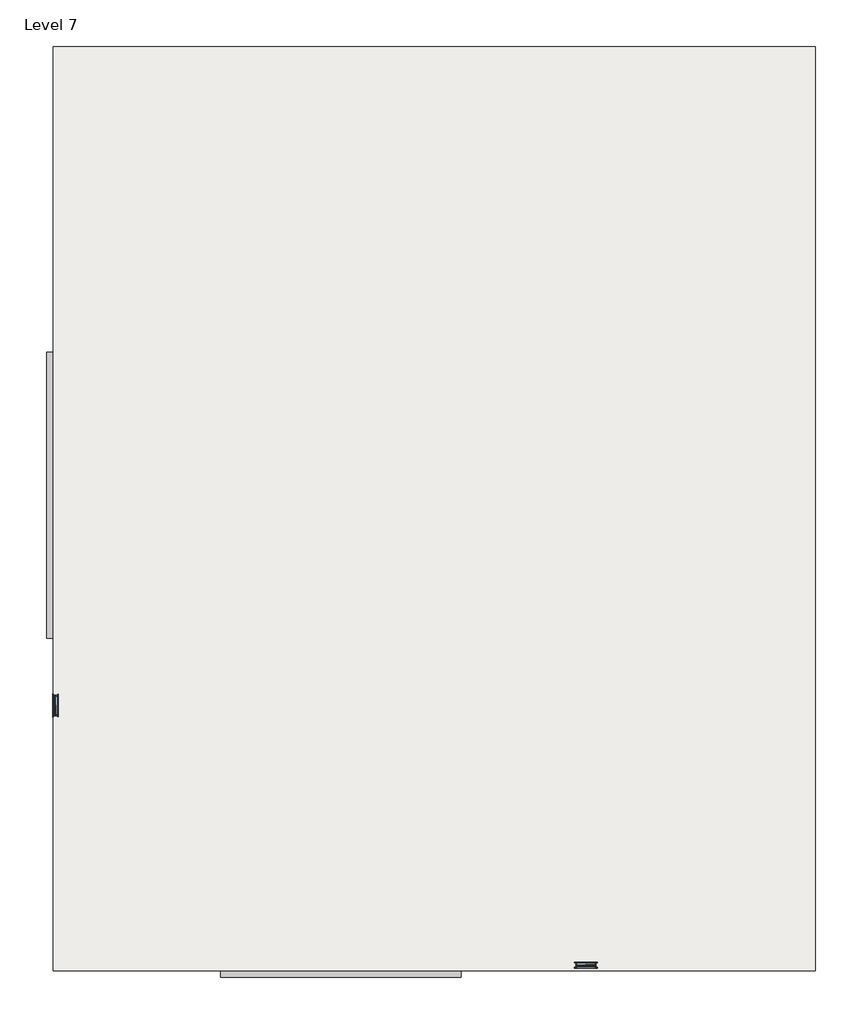
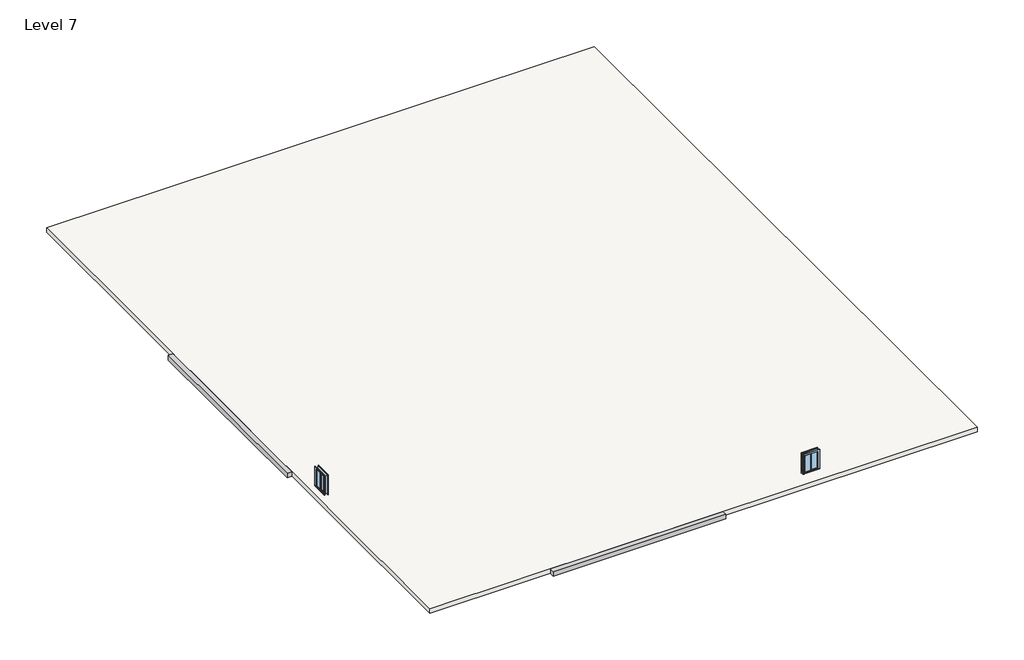
# One storey: 2 proxies, 2 windows, 1 slab.
"""IFC4 building model written with IfcOpenShell, lengths in millimetres."""

from ifc_helpers import new_model, si_unit, frame, origin, place, context, project, spatial, polyline, outline, extrude, transform, mapped, element, save
from components import generic_models_20_generic_models_20_2b057986, generic_models_9_generic_models_9_b7a25faa, window_54100e87

model = new_model("IFC4")

# Units and contexts
model_context = context("Model", 3, world=origin())
ifc_project = project(units=[si_unit("LENGTHUNIT", "METRE", prefix="MILLI")], contexts=[model_context])

# Site, building, storey
site = spatial("IfcSite", under=ifc_project)
building = spatial("IfcBuilding", under=site)
storey = spatial("IfcBuildingStorey", under=building, Name="Level 7", Elevation=12801.6)

# Proxies
placement = place(None, origin())
generic_models_20_generic_models_20_shape = generic_models_20_generic_models_20_2b057986(model_context)
element("IfcBuildingElementProxy", 1, Name="Generic Models 20 : Generic Models 20", ObjectType="Generic Models 20 : Generic Models 20", at=placement, inside=storey, context=model_context, shape_type="MappedRepresentation", body=[
    mapped(generic_models_20_generic_models_20_shape, transform((0.0, 0.0, 0.0), x_axis=(1.0, 0.0, 0.0), y_axis=(0.0, 1.0, 0.0), z_axis=(0.0, 0.0, 1.0))),
])
generic_models_9_generic_models_9_shape = generic_models_9_generic_models_9_b7a25faa(model_context)
element("IfcBuildingElementProxy", 2, Name="Generic Models 9 : Generic Models 9", ObjectType="Generic Models 9 : Generic Models 9", at=placement, inside=storey, context=model_context, shape_type="MappedRepresentation", body=[
    mapped(generic_models_9_generic_models_9_shape, transform((0.0, 0.0, 0.0), x_axis=(1.0, 0.0, 0.0), y_axis=(0.0, 1.0, 0.0), z_axis=(0.0, 0.0, 1.0))),
])

# Slab
element("IfcSlab", 3, ObjectType="Generic - 12\"", at=placement, inside=storey, context=model_context, shape_type="SweptSolid", body=[
    extrude(outline(polyline([(19165.761926, 20759.4014639), (19165.761926, -20998.1985361), (-15276.638074, -20998.1985361), (-15276.638074, 20759.4014639), (19165.761926, 20759.4014639)])), frame((0.0, 0.0, 12801.6), z_axis=(0.0, 0.0, 1.0), x_axis=(1.0, 0.0, 0.0)), (0.0, 0.0, 1.0), 304.8),
])

# Windows
window_shape = window_54100e87(model_context)
element("IfcWindow", 4, ObjectType="Slider with Trim : 36\" x 48\"", at=placement, inside=storey, context=model_context, shape_type="MappedRepresentation", body=[
    mapped(window_shape, transform((8802.561926, -20744.1985361, 12801.6), x_axis=(-1.0, 0.0, 0.0), y_axis=(0.0, -1.0, 0.0), z_axis=(0.0, 0.0, 1.0))),
])
element("IfcWindow", 5, ObjectType="Slider with Trim : 36\" x 48\"", at=placement, inside=storey, context=model_context, shape_type="MappedRepresentation", body=[
    mapped(window_shape, transform((-15175.038074, -9014.8213044, 12801.6), x_axis=(0.0, 1.0, 0.0), y_axis=(-1.0, 0.0, 0.0), z_axis=(0.0, 0.0, 1.0))),
])

save(model, "model.ifc")

# Revit data of these elements
# Type "Generic - 12\""
#   Assembly Code = "B1010"
#   Function = 0
#   Layers, outside or top first: 1' - 0" no material (function 1)
# Type "Slider with Trim : 36\" x 48\""
#   Type Mark = "22"
#   Construction Type Id = "GSP4R"
#   Assembly Code = "B2020100"
#   Analytic Construction = "1/8 in Pilkington single glazing"
#   Visual Light Transmittance = 0.9
#   Solar Heat Gain Coefficient = 0.78
#   Heat Transfer Coefficient (U) = 0.6496 BTU/(h·ft²·°F)
#   Height = 4' - 0"
#   Default Sill Height = 3' - 0"
#   Trim Projection - Ext. = 0' - 0 3/4"
#   Trim Projection - Int. = 0' - 0 3/4"
#   Trim Width - Exterior = 0' - 3 1/2"
#   Trim Width - Interior = 0' - 3 1/2"
#   Width = 3' - 0"
#   Window Inset = 0' - 0 3/4"
#   Define Thermal Properties by = 1
#   Glass Pane Material = Glass
#   Sash Material = Sash
#   Trim Exterior Material = Trim
#   Trim Interior Material = Trim
#   Wall Closure = (empty or 0)
# Element 1 (IfcBuildingElementProxy, "Generic Models 20 : Generic Models 20")
#   Phase Created = New Construction
# Element 2 (IfcBuildingElementProxy, "Generic Models 9 : Generic Models 9")
#   Phase Created = New Construction
# Element 3 (IfcSlab, "Generic - 12\"")
#   Height Offset From Level = 1' - 0"
#   Phase Created = New Construction
#   Materials on its faces: "Default Floor"
# Element 4 (IfcWindow, "Slider with Trim : 36\" x 48\"")
#   Mark = "30"
#   Phase Created = New Construction
#   Materials on its faces: "Sash", "Trim", "Glass"
# Element 5 (IfcWindow, "Slider with Trim : 36\" x 48\"")
#   Mark = "41"
#   Phase Created = New Construction
#   Materials on its faces: "Sash", "Trim", "Glass"
# Materials
#   "Glass": class "Glass", colour RGB 0 128 192, transparency 0.75, Description = "Soda Lime Glass", Cost = 0
#   "Sash": class "Wood", colour RGB 224 178 126, transparency 0
#   "Trim": class "Wood", colour RGB 224 178 126, transparency 0
#   "Default Floor": colour RGB 128 128 128, transparency 0
